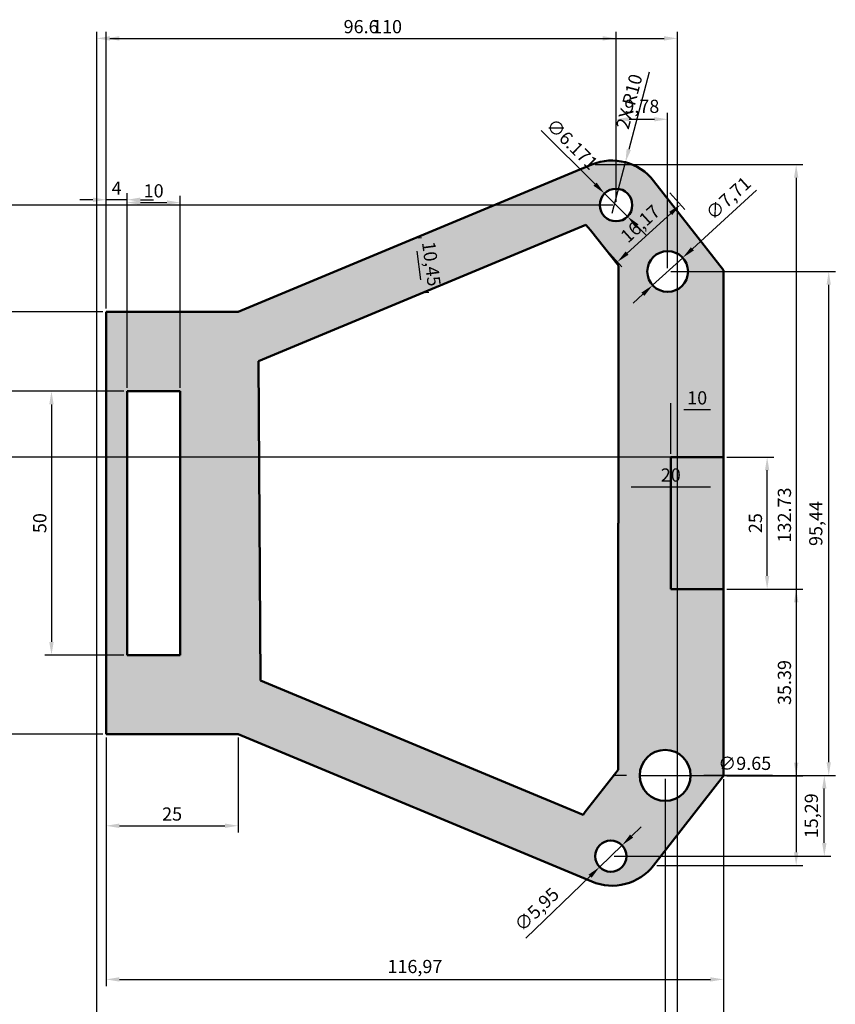
# Model space of a CAD drawing. Units: millimetres. Extents: x 2180 to 2428, y 1025 to 1371.
# Tile 3 of 3: x 2274 to 2428, y 1185 to 1371. Entities that reach past the tile are written whole.
import ezdxf

# ---------------------------------------------------------------- set-up
doc = ezdxf.new("R2010")
doc.units = ezdxf.units.MM
for name, color, linetype, lineweight in [('M-DIMS', 2, 'Continuous', 25), ('M-HATC', 252, 'Continuous', 18), ('M-OUTL', 7, 'Continuous', 50)]:
    doc.layers.add(name, color=color, linetype=linetype, lineweight=lineweight)
doc.styles.get("Standard").update_dxf_attribs({"font": 'arial.ttf'})
doc.dimstyles.new('ISO-25', dxfattribs={"dimtxt": 2.5, "dimasz": 2.5, "dimexe": 1.25, "dimexo": 0.625, "dimtad": 1, "dimtxsty": 'Standard', "dimcen": 2.5, "dimadec": 0, "dimazin": 0, "dimtfac": 1, "dimtmove": 0, "dimatfit": 3, "dimfxl": 1, "dimarcsym": 0})

# ---------------------------------------------------------------- blocks, each defined once
blk = doc.blocks.new('*D6')
at = {"layer": 'Defpoints', "color": 0, "transparency": 16777216}
for p in [(2290.36, 1316.12), (2266.28, 1236.12), (2290.36, 1236.12)]:
    blk.add_point(p, dxfattribs=at)
at = {"layer": 'M-DIMS', "color": 0, "lineweight": -2, "transparency": 16777216}
for p, q in [((2289.74, 1316.12), (2265.03, 1316.12)), ((2266.28, 1313.62), (2266.28, 1238.62)), ((2289.74, 1236.12), (2265.03, 1236.12))]:
    blk.add_line(p, q, dxfattribs=at)
at = {"layer": 'M-DIMS', "color": 0, "transparency": 16777216}
for points in [[(2265.87, 1313.62), (2266.7, 1313.62), (2266.28, 1316.12)], [(2265.87, 1238.62), (2266.7, 1238.62), (2266.28, 1236.12)]]:
    blk.add_solid(points, dxfattribs=at)
at = {"layer": 'M-DIMS', "color": 0, "transparency": 16777216, "insert": (2264.38, 1276.12), "char_height": 2.5, "attachment_point": 5, "rotation": 90}
blk.add_mtext('80', dxfattribs=at)
blk = doc.blocks.new('*D7')
at = {"layer": 'Defpoints', "color": 0, "transparency": 16777216}
for p in [(2294.36, 1301.12), (2280.01, 1251.12), (2294.36, 1251.12)]:
    blk.add_point(p, dxfattribs=at)
at = {"layer": 'M-DIMS', "color": 0, "lineweight": -2, "transparency": 16777216}
for p, q in [((2293.74, 1301.12), (2278.76, 1301.12)), ((2280.01, 1298.62), (2280.01, 1253.62)), ((2293.74, 1251.12), (2278.76, 1251.12))]:
    blk.add_line(p, q, dxfattribs=at)
at = {"layer": 'M-DIMS', "color": 0, "transparency": 16777216}
for points in [[(2279.59, 1298.62), (2280.42, 1298.62), (2280.01, 1301.12)], [(2279.59, 1253.62), (2280.42, 1253.62), (2280.01, 1251.12)]]:
    blk.add_solid(points, dxfattribs=at)
at = {"layer": 'M-DIMS', "color": 0, "transparency": 16777216, "insert": (2278.11, 1276.12), "char_height": 2.5, "attachment_point": 5, "rotation": 90}
blk.add_mtext('50', dxfattribs=at)
blk = doc.blocks.new('*D8')
at = {"layer": 'Defpoints', "color": 0, "transparency": 16777216}
for p in [(2290.36, 1337.37), (2290.36, 1316.12), (2294.36, 1301.12)]:
    blk.add_point(p, dxfattribs=at)
at = {"layer": 'M-DIMS', "color": 0, "lineweight": -2, "transparency": 16777216}
for p, q in [((2287.86, 1337.37), (2285.36, 1337.37)), ((2290.36, 1316.75), (2290.36, 1338.62)), ((2294.36, 1337.37), (2290.36, 1337.37)), ((2294.36, 1301.75), (2294.36, 1338.62)), ((2296.86, 1337.37), (2299.36, 1337.37))]:
    blk.add_line(p, q, dxfattribs=at)
at = {"layer": 'M-DIMS', "color": 0, "transparency": 16777216}
for points in [[(2287.86, 1337.79), (2287.86, 1336.95), (2290.36, 1337.37)], [(2296.86, 1337.79), (2296.86, 1336.95), (2294.36, 1337.37)]]:
    blk.add_solid(points, dxfattribs=at)
at = {"layer": 'M-DIMS', "color": 0, "transparency": 16777216, "insert": (2292.36, 1339.25), "char_height": 2.5, "attachment_point": 5}
blk.add_mtext('4', dxfattribs=at)
blk = doc.blocks.new('*D9')
at = {"layer": 'Defpoints', "color": 0, "transparency": 16777216}
for p in [(2304.36, 1336.83), (2294.36, 1301.12), (2304.36, 1301.12)]:
    blk.add_point(p, dxfattribs=at)
at = {"layer": 'M-DIMS', "color": 0, "lineweight": -2, "transparency": 16777216}
for p, q in [((2294.36, 1301.75), (2294.36, 1338.08)), ((2304.36, 1301.75), (2304.36, 1338.08)), ((2296.86, 1336.83), (2301.86, 1336.83))]:
    blk.add_line(p, q, dxfattribs=at)
at = {"layer": 'M-DIMS', "color": 0, "transparency": 16777216}
for points in [[(2296.86, 1337.25), (2296.86, 1336.42), (2294.36, 1336.83)], [(2301.86, 1337.25), (2301.86, 1336.42), (2304.36, 1336.83)]]:
    blk.add_solid(points, dxfattribs=at)
at = {"layer": 'M-DIMS', "color": 0, "transparency": 16777216, "insert": (2299.36, 1338.73), "char_height": 2.5, "attachment_point": 5}
blk.add_mtext('10', dxfattribs=at)
blk = doc.blocks.new('*D10')
at = {"layer": 'Defpoints', "color": 0, "transparency": 16777216}
for p in [(2348.86, 1330.08), (2350.25, 1319.72), (2350.25, 1319.72)]:
    blk.add_point(p, dxfattribs=at)
at = {"layer": 'M-DIMS', "color": 0, "lineweight": -2, "transparency": 16777216}
for p, q in [((2349.48, 1330.16), (2350.1, 1330.24)), ((2349.19, 1327.6), (2349.92, 1322.2)), ((2350.87, 1319.81), (2351.49, 1319.89))]:
    blk.add_line(p, q, dxfattribs=at)
at = {"layer": 'M-DIMS', "color": 0, "transparency": 16777216}
for points in [[(2349.61, 1327.65), (2348.78, 1327.54), (2348.86, 1330.08)], [(2350.33, 1322.26), (2349.5, 1322.14), (2350.25, 1319.72)]]:
    blk.add_solid(points, dxfattribs=at)
at = {"layer": 'M-DIMS', "color": 0, "transparency": 16777216, "insert": (2351.66, 1325.18), "char_height": 2.5, "attachment_point": 5, "rotation": 277.6268}
blk.add_mtext('10,45', dxfattribs=at)
blk = doc.blocks.new('*D11')
at = {"layer": 'Defpoints', "color": 0, "transparency": 16777216}
for p in [(2290.36, 1236.12), (2315.36, 1236.12), (2315.36, 1218.8)]:
    blk.add_point(p, dxfattribs=at)
at = {"layer": 'M-DIMS', "color": 0, "lineweight": -2, "transparency": 16777216}
for p, q in [((2290.36, 1235.5), (2290.36, 1217.55)), ((2315.36, 1235.5), (2315.36, 1217.55)), ((2292.86, 1218.8), (2312.86, 1218.8))]:
    blk.add_line(p, q, dxfattribs=at)
at = {"layer": 'M-DIMS', "color": 0, "transparency": 16777216}
for points in [[(2292.86, 1219.22), (2292.86, 1218.38), (2290.36, 1218.8)], [(2312.86, 1219.22), (2312.86, 1218.38), (2315.36, 1218.8)]]:
    blk.add_solid(points, dxfattribs=at)
at = {"layer": 'M-DIMS', "color": 0, "transparency": 16777216, "insert": (2302.86, 1220.7), "char_height": 2.5, "attachment_point": 5}
blk.add_mtext('25', dxfattribs=at)
blk = doc.blocks.new('*D12')
at = {"layer": 'Defpoints', "color": 0, "transparency": 16777216}
for p in [(2290.36, 1236.12), (2407.33, 1228.24), (2407.33, 1189.7)]:
    blk.add_point(p, dxfattribs=at)
at = {"layer": 'M-DIMS', "color": 0, "lineweight": -2, "transparency": 16777216}
for p, q in [((2290.36, 1235.5), (2290.36, 1188.45)), ((2407.33, 1227.61), (2407.33, 1188.45)), ((2292.86, 1189.7), (2404.83, 1189.7))]:
    blk.add_line(p, q, dxfattribs=at)
at = {"layer": 'M-DIMS', "color": 0, "transparency": 16777216}
for points in [[(2292.86, 1190.11), (2292.86, 1189.28), (2290.36, 1189.7)], [(2404.83, 1190.11), (2404.83, 1189.28), (2407.33, 1189.7)]]:
    blk.add_solid(points, dxfattribs=at)
at = {"layer": 'M-DIMS', "color": 0, "transparency": 16777216, "insert": (2348.85, 1191.82), "char_height": 2.5, "attachment_point": 5}
blk.add_mtext('116,97', dxfattribs=at)
blk = doc.blocks.new('*D13')
at = {"layer": 'Defpoints', "color": 0, "transparency": 16777216}
for p in [(2396.26, 1228.33), (2426.41, 1228.33), (2385.97, 1213.04)]:
    blk.add_point(p, dxfattribs=at)
at = {"layer": 'M-DIMS', "color": 0, "lineweight": -2, "transparency": 16777216}
for p, q in [((2396.89, 1228.33), (2427.66, 1228.33)), ((2426.41, 1215.54), (2426.41, 1225.83)), ((2386.59, 1213.04), (2427.66, 1213.04))]:
    blk.add_line(p, q, dxfattribs=at)
at = {"layer": 'M-DIMS', "color": 0, "transparency": 16777216}
for points in [[(2425.99, 1225.83), (2426.83, 1225.83), (2426.41, 1228.33)], [(2425.99, 1215.54), (2426.83, 1215.54), (2426.41, 1213.04)]]:
    blk.add_solid(points, dxfattribs=at)
at = {"layer": 'M-DIMS', "color": 0, "transparency": 16777216, "insert": (2424.28, 1220.69), "char_height": 2.5, "attachment_point": 5, "rotation": 90}
blk.add_mtext('15,29', dxfattribs=at)
blk = doc.blocks.new('*D14')
at = {"layer": 'Defpoints', "color": 0, "transparency": 16777216}
for p in [(2396.73, 1323.77), (2427.25, 1323.77), (2396.26, 1228.33)]:
    blk.add_point(p, dxfattribs=at)
at = {"layer": 'M-DIMS', "color": 0, "lineweight": -2, "transparency": 16777216}
for p, q in [((2397.36, 1323.77), (2428.5, 1323.77)), ((2427.25, 1230.83), (2427.25, 1321.27)), ((2396.89, 1228.33), (2428.5, 1228.33))]:
    blk.add_line(p, q, dxfattribs=at)
at = {"layer": 'M-DIMS', "color": 0, "transparency": 16777216}
for points in [[(2426.83, 1321.27), (2427.66, 1321.27), (2427.25, 1323.77)], [(2426.83, 1230.83), (2427.66, 1230.83), (2427.25, 1228.33)]]:
    blk.add_solid(points, dxfattribs=at)
at = {"layer": 'M-DIMS', "color": 0, "transparency": 16777216, "insert": (2425.12, 1276.05), "char_height": 2.5, "attachment_point": 5, "rotation": 90}
blk.add_mtext('95,44', dxfattribs=at)
blk = doc.blocks.new('*D15')
at = {"layer": 'Defpoints', "color": 0, "transparency": 16777216}
for p in [(2396.73, 1352.61), (2386.95, 1336.37), (2396.73, 1323.77)]:
    blk.add_point(p, dxfattribs=at)
at = {"layer": 'M-DIMS', "color": 0, "lineweight": -2, "transparency": 16777216}
for p, q in [((2386.95, 1337), (2386.95, 1353.86)), ((2389.45, 1352.61), (2394.23, 1352.61)), ((2396.73, 1324.4), (2396.73, 1353.86))]:
    blk.add_line(p, q, dxfattribs=at)
at = {"layer": 'M-DIMS', "color": 0, "transparency": 16777216}
for points in [[(2389.45, 1353.03), (2389.45, 1352.2), (2386.95, 1352.61)], [(2394.23, 1353.03), (2394.23, 1352.2), (2396.73, 1352.61)]]:
    blk.add_solid(points, dxfattribs=at)
at = {"layer": 'M-DIMS', "color": 0, "transparency": 16777216, "insert": (2391.84, 1354.74), "char_height": 2.5, "attachment_point": 5}
blk.add_mtext('9,78', dxfattribs=at)
blk = doc.blocks.new('*D16')
at = {"layer": 'Defpoints', "color": 0, "transparency": 16777216}
for p in [(2399.58, 1326.38), (2393.89, 1321.17)]:
    blk.add_point(p, dxfattribs=at)
at = {"layer": 'M-DIMS', "color": 0, "lineweight": -2, "transparency": 16777216}
for p, q in [((2413.59, 1339.2), (2401.42, 1328.06)), ((2393.89, 1321.17), (2399.58, 1326.38)), ((2392.04, 1319.48), (2390.2, 1317.79))]:
    blk.add_line(p, q, dxfattribs=at)
at = {"layer": 'M-DIMS', "color": 0, "transparency": 16777216}
for points in [[(2401.14, 1328.37), (2401.7, 1327.76), (2399.58, 1326.38)], [(2391.76, 1319.79), (2392.33, 1319.17), (2393.89, 1321.17)]]:
    blk.add_solid(points, dxfattribs=at)
at = {"layer": 'M-DIMS', "color": 0, "transparency": 16777216, "insert": (2408.44, 1337.43), "char_height": 2.5, "attachment_point": 5, "rotation": 42.4638}
blk.add_mtext('∅7,71', dxfattribs=at)
blk = doc.blocks.new('*D17')
at = {"layer": 'Defpoints', "color": 0, "transparency": 16777216}
for p in [(2388.11, 1215.11), (2383.83, 1210.98)]:
    blk.add_point(p, dxfattribs=at)
at = {"layer": 'M-DIMS', "color": 0, "lineweight": -2, "transparency": 16777216}
for p, q in [((2389.9, 1216.84), (2391.7, 1218.58)), ((2388.11, 1215.11), (2383.83, 1210.98)), ((2369.88, 1197.52), (2382.03, 1209.24))]:
    blk.add_line(p, q, dxfattribs=at)
at = {"layer": 'M-DIMS', "color": 0, "transparency": 16777216}
for points in [[(2389.61, 1217.14), (2390.19, 1216.54), (2388.11, 1215.11)], [(2381.74, 1209.54), (2382.32, 1208.94), (2383.83, 1210.98)]]:
    blk.add_solid(points, dxfattribs=at)
at = {"layer": 'M-DIMS', "color": 0, "transparency": 16777216, "insert": (2372.15, 1202.72), "char_height": 2.5, "attachment_point": 5, "rotation": 43.9913}
blk.add_mtext('∅5,95', dxfattribs=at)
blk = doc.blocks.new('*D18')
at = {"layer": 'Defpoints', "color": 0, "transparency": 16777216}
for p in [(2407.33, 1283.01), (2387.33, 1276.12), (2407.33, 1276.12)]:
    blk.add_point(p, dxfattribs=at)
at = {"layer": 'M-DIMS', "color": 0, "lineweight": -2, "transparency": 16777216}
for p, q in [((2387.33, 1276.75), (2387.33, 1284.26)), ((2407.33, 1276.75), (2407.33, 1284.26)), ((2389.83, 1283.01), (2404.83, 1283.01))]:
    blk.add_line(p, q, dxfattribs=at)
at = {"layer": 'M-DIMS', "color": 0, "transparency": 16777216}
for points in [[(2389.83, 1283.42), (2389.83, 1282.59), (2387.33, 1283.01)], [(2404.83, 1283.42), (2404.83, 1282.59), (2407.33, 1283.01)]]:
    blk.add_solid(points, dxfattribs=at)
at = {"layer": 'M-DIMS', "color": 0, "transparency": 16777216, "insert": (2397.33, 1284.91), "char_height": 2.5, "attachment_point": 5}
blk.add_mtext('20', dxfattribs=at)
blk = doc.blocks.new('*D19')
at = {"layer": 'Defpoints', "color": 0, "transparency": 16777216}
for p in [(2396.73, 1339.13), (2399.16, 1336.46), (2384.77, 1328.26)]:
    blk.add_point(p, dxfattribs=at)
at = {"layer": 'M-DIMS', "color": 0, "lineweight": -2, "transparency": 16777216}
for p, q in [((2397.15, 1338.67), (2400, 1335.53)), ((2389.05, 1327.27), (2397.31, 1334.78)), ((2385.19, 1327.79), (2388.04, 1324.66))]:
    blk.add_line(p, q, dxfattribs=at)
at = {"layer": 'M-DIMS', "color": 0, "transparency": 16777216}
for points in [[(2397.03, 1335.08), (2397.59, 1334.47), (2399.16, 1336.46)], [(2388.77, 1327.57), (2389.33, 1326.96), (2387.2, 1325.58)]]:
    blk.add_solid(points, dxfattribs=at)
at = {"layer": 'M-DIMS', "color": 0, "transparency": 16777216, "insert": (2391.75, 1332.59), "char_height": 2.5, "attachment_point": 5, "rotation": 42.2758}
blk.add_mtext('16,17', dxfattribs=at)
blk = doc.blocks.new('*D20')
at = {"layer": 'Defpoints', "color": 0, "transparency": 16777216}
for p in [(2407.33, 1288.62), (2415.58, 1288.62), (2407.33, 1263.62)]:
    blk.add_point(p, dxfattribs=at)
at = {"layer": 'M-DIMS', "color": 0, "lineweight": -2, "transparency": 16777216}
for p, q in [((2407.96, 1288.62), (2416.83, 1288.62)), ((2415.58, 1266.12), (2415.58, 1286.12)), ((2407.96, 1263.62), (2416.83, 1263.62))]:
    blk.add_line(p, q, dxfattribs=at)
at = {"layer": 'M-DIMS', "color": 0, "transparency": 16777216}
for points in [[(2415.16, 1286.12), (2415.99, 1286.12), (2415.58, 1288.62)], [(2415.16, 1266.12), (2415.99, 1266.12), (2415.58, 1263.62)]]:
    blk.add_solid(points, dxfattribs=at)
at = {"layer": 'M-DIMS', "color": 0, "transparency": 16777216, "insert": (2413.68, 1276.12), "char_height": 2.5, "attachment_point": 5, "rotation": 90}
blk.add_mtext('25', dxfattribs=at)
blk = doc.blocks.new('*D21')
at = {"layer": 'Defpoints', "color": 0, "transparency": 16777216}
for p in [(2407.33, 1297.62), (2397.33, 1288.62), (2407.33, 1288.62)]:
    blk.add_point(p, dxfattribs=at)
at = {"layer": 'M-DIMS', "color": 0, "lineweight": -2, "transparency": 16777216}
for p, q in [((2397.33, 1289.25), (2397.33, 1298.87)), ((2407.33, 1289.25), (2407.33, 1298.87)), ((2399.83, 1297.62), (2404.83, 1297.62))]:
    blk.add_line(p, q, dxfattribs=at)
at = {"layer": 'M-DIMS', "color": 0, "transparency": 16777216}
for points in [[(2399.83, 1298.04), (2399.83, 1297.2), (2397.33, 1297.62)], [(2404.83, 1298.04), (2404.83, 1297.2), (2407.33, 1297.62)]]:
    blk.add_solid(points, dxfattribs=at)
at = {"layer": 'M-DIMS', "color": 0, "transparency": 16777216, "insert": (2402.33, 1299.52), "char_height": 2.5, "attachment_point": 5}
blk.add_mtext('10', dxfattribs=at)
blk = doc.blocks.new('*D35')
at = {"layer": 'Defpoints', "color": 0, "transparency": 16777216}
for p in [(2386.95, 1367.93), (2386.95, 1336.37), (2290.36, 1316.12)]:
    blk.add_point(p, dxfattribs=at)
at = {"layer": 'M-DIMS', "color": 0, "lineweight": -2, "transparency": 16777216}
for p, q in [((2290.36, 1316.75), (2290.36, 1369.18)), ((2386.95, 1337), (2386.95, 1369.18)), ((2292.86, 1367.93), (2384.45, 1367.93))]:
    blk.add_line(p, q, dxfattribs=at)
at = {"layer": 'M-DIMS', "color": 0, "transparency": 16777216}
for points in [[(2292.86, 1368.35), (2292.86, 1367.51), (2290.36, 1367.93)], [(2384.45, 1368.35), (2384.45, 1367.51), (2386.95, 1367.93)]]:
    blk.add_solid(points, dxfattribs=at)
at = {"layer": 'M-DIMS', "color": 0, "transparency": 16777216, "insert": (2338.66, 1369.83), "char_height": 2.5, "attachment_point": 5}
blk.add_mtext('96.6', dxfattribs=at)
blk = doc.blocks.new('*D36')
at = {"layer": 'Defpoints', "color": 0, "transparency": 16777216}
for p in [(2386.95, 1336.37), (2187.07, 1288.62), (2407.33, 1288.62)]:
    blk.add_point(p, dxfattribs=at)
at = {"layer": 'M-DIMS', "color": 0, "lineweight": -2, "transparency": 16777216}
for p, q in [((2386.33, 1336.37), (2185.82, 1336.37)), ((2187.07, 1333.87), (2187.07, 1291.12)), ((2406.71, 1288.62), (2185.82, 1288.62))]:
    blk.add_line(p, q, dxfattribs=at)
at = {"layer": 'M-DIMS', "color": 0, "transparency": 16777216}
for points in [[(2186.65, 1333.87), (2187.49, 1333.87), (2187.07, 1336.37)], [(2186.65, 1291.12), (2187.49, 1291.12), (2187.07, 1288.62)]]:
    blk.add_solid(points, dxfattribs=at)
at = {"layer": 'M-DIMS', "color": 0, "transparency": 16777216, "insert": (2185.17, 1312.5), "char_height": 2.5, "attachment_point": 5, "rotation": 90}
blk.add_mtext('47.75', dxfattribs=at)
blk = doc.blocks.new('*D37')
at = {"layer": 'Defpoints', "color": 0, "transparency": 16777216}
for p in [(2396.26, 1228.33), (2407.33, 1228.24), (2407.33, 1089.54)]:
    blk.add_point(p, dxfattribs=at)
at = {"layer": 'M-DIMS', "color": 0, "lineweight": -2, "transparency": 16777216}
for p, q in [((2396.26, 1227.71), (2396.26, 1088.29)), ((2407.33, 1227.61), (2407.33, 1088.29)), ((2398.76, 1089.54), (2404.83, 1089.54))]:
    blk.add_line(p, q, dxfattribs=at)
at = {"layer": 'M-DIMS', "color": 0, "transparency": 16777216}
for points in [[(2398.76, 1089.96), (2398.76, 1089.12), (2396.26, 1089.54)], [(2404.83, 1089.96), (2404.83, 1089.12), (2407.33, 1089.54)]]:
    blk.add_solid(points, dxfattribs=at)
at = {"layer": 'M-DIMS', "color": 0, "transparency": 16777216, "insert": (2401.8, 1091.44), "char_height": 2.5, "attachment_point": 5}
blk.add_mtext('11.07', dxfattribs=at)
blk = doc.blocks.new('*D38')
at = {"layer": 'Defpoints', "color": 0, "transparency": 16777216}
for p in [(2407.33, 1263.62), (2407.33, 1228.24), (2421.08, 1228.24)]:
    blk.add_point(p, dxfattribs=at)
at = {"layer": 'M-DIMS', "color": 0, "lineweight": -2, "transparency": 16777216}
for p, q in [((2407.96, 1263.62), (2422.33, 1263.62)), ((2421.08, 1261.12), (2421.08, 1230.74)), ((2407.96, 1228.24), (2422.33, 1228.24))]:
    blk.add_line(p, q, dxfattribs=at)
at = {"layer": 'M-DIMS', "color": 0, "transparency": 16777216}
for points in [[(2420.67, 1261.12), (2421.5, 1261.12), (2421.08, 1263.62)], [(2420.67, 1230.74), (2421.5, 1230.74), (2421.08, 1228.24)]]:
    blk.add_solid(points, dxfattribs=at)
at = {"layer": 'M-DIMS', "color": 0, "transparency": 16777216, "insert": (2419.18, 1245.93), "char_height": 2.5, "attachment_point": 5, "rotation": 90}
blk.add_mtext('35.39', dxfattribs=at)
blk = doc.blocks.new('*D39')
at = {"layer": 'Defpoints', "color": 0, "transparency": 16777216}
for p in [(2382.36, 1344.03), (2394.08, 1211.29), (2421.08, 1211.29)]:
    blk.add_point(p, dxfattribs=at)
at = {"layer": 'M-DIMS', "color": 0, "lineweight": -2, "transparency": 16777216}
for p, q in [((2382.99, 1344.03), (2422.33, 1344.03)), ((2421.08, 1341.53), (2421.08, 1213.79)), ((2394.71, 1211.29), (2422.33, 1211.29))]:
    blk.add_line(p, q, dxfattribs=at)
at = {"layer": 'M-DIMS', "color": 0, "transparency": 16777216}
for points in [[(2420.67, 1341.53), (2421.5, 1341.53), (2421.08, 1344.03)], [(2420.67, 1213.79), (2421.5, 1213.79), (2421.08, 1211.29)]]:
    blk.add_solid(points, dxfattribs=at)
at = {"layer": 'M-DIMS', "color": 0, "transparency": 16777216, "insert": (2419.18, 1277.66), "char_height": 2.5, "attachment_point": 5, "rotation": 90}
blk.add_mtext('132.73', dxfattribs=at)
blk = doc.blocks.new('*D40')
at = {"layer": 'Defpoints', "color": 0, "transparency": 16777216}
for p in [(2290.36, 1316.12), (2187.07, 1301.12), (2294.36, 1301.12)]:
    blk.add_point(p, dxfattribs=at)
at = {"layer": 'M-DIMS', "color": 0, "lineweight": -2, "transparency": 16777216}
for p, q in [((2289.74, 1316.12), (2185.82, 1316.12)), ((2187.07, 1313.62), (2187.07, 1303.62)), ((2293.74, 1301.12), (2185.82, 1301.12))]:
    blk.add_line(p, q, dxfattribs=at)
at = {"layer": 'M-DIMS', "color": 0, "transparency": 16777216}
for points in [[(2186.65, 1313.62), (2187.49, 1313.62), (2187.07, 1316.12)], [(2186.65, 1303.62), (2187.49, 1303.62), (2187.07, 1301.12)]]:
    blk.add_solid(points, dxfattribs=at)
at = {"layer": 'M-DIMS', "color": 0, "transparency": 16777216, "insert": (2185.17, 1308.62), "char_height": 2.5, "attachment_point": 5, "rotation": 90}
blk.add_mtext('15', dxfattribs=at)
blk = doc.blocks.new('*D41')
at = {"layer": 'Defpoints', "color": 0, "transparency": 16777216}
for p in [(2398.57, 1367.93), (2288.57, 1149.5), (2398.57, 1149.5)]:
    blk.add_point(p, dxfattribs=at)
at = {"layer": 'M-DIMS', "color": 0, "lineweight": -2, "transparency": 16777216}
for p, q in [((2288.57, 1150.12), (2288.57, 1369.18)), ((2398.57, 1150.12), (2398.57, 1369.18)), ((2291.07, 1367.93), (2396.07, 1367.93))]:
    blk.add_line(p, q, dxfattribs=at)
at = {"layer": 'M-DIMS', "color": 0, "transparency": 16777216}
for points in [[(2291.07, 1368.35), (2291.07, 1367.51), (2288.57, 1367.93)], [(2396.07, 1368.35), (2396.07, 1367.51), (2398.57, 1367.93)]]:
    blk.add_solid(points, dxfattribs=at)
at = {"layer": 'M-DIMS', "color": 0, "transparency": 16777216, "insert": (2343.57, 1369.83), "char_height": 2.5, "attachment_point": 5}
blk.add_mtext('110', dxfattribs=at)
blk = doc.blocks.new('*D48')
at = {"layer": 'Defpoints', "color": 0, "transparency": 16777216}
for p in [(2388.74, 1344.47), (2386.21, 1334.8)]:
    blk.add_point(p, dxfattribs=at)
at = {"layer": 'M-DIMS', "color": 0, "lineweight": -2, "transparency": 16777216}
for p, q in [((2393.21, 1361.52), (2389.37, 1346.89)), ((2386.21, 1334.8), (2388.74, 1344.47))]:
    blk.add_line(p, q, dxfattribs=at)
at = {"layer": 'M-DIMS', "color": 0, "transparency": 16777216}
blk.add_solid([(2388.97, 1346.99), (2389.78, 1346.78), (2388.74, 1344.47)], dxfattribs=at)
at = {"layer": 'M-DIMS', "color": 0, "transparency": 16777216, "insert": (2389.77, 1355.9), "char_height": 2.5, "attachment_point": 5, "rotation": 75.3136}
blk.add_mtext('2X R10', dxfattribs=at)
blk = doc.blocks.new('*D49')
at = {"layer": 'Defpoints', "color": 0, "transparency": 16777216}
for p in [(2391.44, 1228.33), (2401.09, 1228.33)]:
    blk.add_point(p, dxfattribs=at)
at = {"layer": 'M-DIMS', "color": 0, "lineweight": -2, "transparency": 16777216}
for p, q in [((2388.94, 1228.33), (2386.44, 1228.33)), ((2391.44, 1228.33), (2401.09, 1228.33)), ((2416.57, 1228.33), (2403.59, 1228.33))]:
    blk.add_line(p, q, dxfattribs=at)
at = {"layer": 'M-DIMS', "color": 0, "transparency": 16777216}
for points in [[(2388.94, 1228.75), (2388.94, 1227.91), (2391.44, 1228.33)], [(2403.59, 1228.75), (2403.59, 1227.91), (2401.09, 1228.33)]]:
    blk.add_solid(points, dxfattribs=at)
at = {"layer": 'M-DIMS', "color": 0, "transparency": 16777216, "insert": (2411.33, 1230.3), "char_height": 2.5, "attachment_point": 5, "rotation": 359.9984}
blk.add_mtext('∅9.65', dxfattribs=at)
blk = doc.blocks.new('*D50')
at = {"layer": 'Defpoints', "color": 0, "transparency": 16777216}
for p in [(2384.77, 1338.55), (2389.14, 1334.19)]:
    blk.add_point(p, dxfattribs=at)
at = {"layer": 'M-DIMS', "color": 0, "lineweight": -2, "transparency": 16777216}
for p, q in [((2372.79, 1350.5), (2383, 1340.32)), ((2389.14, 1334.19), (2384.77, 1338.55)), ((2390.91, 1332.43), (2392.68, 1330.66))]:
    blk.add_line(p, q, dxfattribs=at)
at = {"layer": 'M-DIMS', "color": 0, "transparency": 16777216}
for points in [[(2383.29, 1340.61), (2382.7, 1340.02), (2384.77, 1338.55)], [(2391.2, 1332.72), (2390.61, 1332.13), (2389.14, 1334.19)]]:
    blk.add_solid(points, dxfattribs=at)
at = {"layer": 'M-DIMS', "color": 0, "transparency": 16777216, "insert": (2378.4, 1347.69), "char_height": 2.5, "attachment_point": 5, "rotation": 315.0756}
blk.add_mtext('∅6.171', dxfattribs=at)

msp = doc.modelspace()

# ---------------------------------------------------------------- hatches: boundary and pattern name
at = {"layer": 'M-HATC'}
h = msp.add_hatch(color=256, dxfattribs=at)
h.set_gradient(color1=(100, 33, 101), color2=(100, 33, 101), tint=1)
h.paths.add_polyline_path([(2290.3614, 1316.125), (2290.3614, 1236.125), (2315.3614, 1236.125), (2382.3613, 1208.2225, 0.33744335), (2394.0834, 1211.2942), (2407.3324, 1228.2381), (2407.3324, 1276.125), (2407.3324, 1324.0118), (2394.0834, 1340.9557, 0.33744335), (2382.3613, 1344.0274), (2315.3614, 1316.125)])
h.paths.add_polyline_path([(2304.3614, 1301.125), (2304.3614, 1251.125), (2294.3614, 1251.125), (2294.3614, 1301.125)], flags=16)
h.paths.add_polyline_path([(2319.2409, 1306.8094), (2381.2546, 1332.6353), (2382.1426, 1331.6188), (2387.4019, 1324.8927), (2387.4019, 1324.0118), (2387.4019, 1276.125), (2387.3338, 1229.3759), (2381.1207, 1221.4302), (2380.7182, 1220.8933), (2319.6154, 1246.3398)], flags=16)
h.paths.add_polyline_path([(2383.8679, 1336.3721, -1), (2390.0393, 1336.3721, -1)], flags=16)
h.paths.add_polyline_path([(2392.8764, 1323.7723, -1), (2400.5906, 1323.7723, -1)], flags=16)
h.paths.add_polyline_path([(2401.0881, 1228.3311, -1), (2391.4386, 1228.3311, -1)], flags=16)
h.paths.add_polyline_path([(2388.94, 1213.0425, -1), (2382.9912, 1213.0425, -1)], flags=16)

# ---------------------------------------------------------------- linework, layer by layer
at = {"layer": 'M-OUTL'}
for p, q in [((2315.3614, 1316.125), (2382.3613, 1344.0274)), ((2394.0834, 1340.9557), (2407.3324, 1324.0118)), ((2319.2409, 1306.8094), (2381.2546, 1332.6353)), ((2382.1426, 1331.6188), (2381.2546, 1332.6353)), ((2382.1426, 1331.6188), (2387.4019, 1324.8927)), ((2387.4019, 1324.0118), (2387.4019, 1324.8927)), ((2387.4019, 1324.0118), (2387.4019, 1276.125)), ((2407.3324, 1324.0118), (2407.3324, 1276.125)), ((2290.3614, 1316.125), (2290.3614, 1236.125)), ((2290.3614, 1316.125), (2315.3614, 1316.125)), ((2319.2409, 1306.8094), (2319.6154, 1246.3398)), ((2294.3614, 1301.125), (2294.3614, 1251.125)), ((2304.3614, 1301.125), (2294.3614, 1301.125)), ((2304.3614, 1251.125), (2304.3614, 1301.125)), ((2407.3324, 1288.625), (2397.3324, 1288.625)), ((2397.3324, 1288.625), (2397.3324, 1263.625)), ((2407.3324, 1276.125), (2407.3324, 1288.625)), ((2387.3338, 1229.3759), (2387.3338, 1276.125)), ((2407.3324, 1228.2381), (2407.3324, 1276.125)), ((2397.3324, 1263.625), (2407.3324, 1263.625)), ((2294.3614, 1251.125), (2304.3614, 1251.125)), ((2319.6154, 1246.3398), (2380.7182, 1220.8933)), ((2290.3614, 1236.125), (2315.3614, 1236.125)), ((2315.3614, 1236.125), (2382.3613, 1208.2225)), ((2381.1207, 1221.4302), (2387.3338, 1229.3759)), ((2394.0834, 1211.2942), (2407.3324, 1228.2381)), ((2381.1207, 1221.4302), (2380.7182, 1220.8933))]:
    msp.add_line(p, q, dxfattribs=at)
for centre, radius in [((2386.9536, 1336.3721), 3.0857), ((2396.7335, 1323.7723), 3.8571), ((2396.2634, 1228.3311), 4.8247), ((2385.9656, 1213.0425), 2.9744)]:
    msp.add_circle(centre, radius, dxfattribs=at)
for centre, start, end in [((2386.2058, 1334.7959), 38.023033, 112.609533), ((2386.2058, 1217.454), 247.390467, 321.976967)]:
    msp.add_arc(centre, 10, start, end, dxfattribs=at)

# ---------------------------------------------------------------- dimensions: what is measured, and where the dimension line sits
at = {"layer": 'M-DIMS'}
for base, p1, p2, override, picture, middle in [((2398.5713, 1367.9295), (2288.5713, 1149.4968), (2398.5713, 1149.4968), {"dimdec": 0, "dimlfac": 1, "dimrnd": 0, "dimzin": 0, "dimdsep": 46, "dimlunit": 2}, '*D41', (2343.5713, 1369.831)), ((2386.9536, 1367.9295), (2290.3614, 1316.125), (2386.9536, 1336.3721), {"dimdec": 1, "dimlfac": 1, "dimrnd": 0, "dimzin": 0, "dimdsep": 46, "dimlunit": 2}, '*D35', (2338.6575, 1369.831)), ((2396.7335, 1352.6134), (2386.9536, 1336.3721), (2396.7335, 1323.7723), {"dimclrd": 0, "dimclre": 0, "dimclrt": 0}, '*D15', (2391.8435, 1354.7408)), ((2290.3614, 1337.3704), (2294.3614, 1301.125), (2290.3614, 1316.125), {"dimclrd": 0, "dimclre": 0, "dimclrt": 0}, '*D8', (2292.3614, 1339.2454)), ((2304.3614, 1336.8327), (2294.3614, 1301.125), (2304.3614, 1301.125), {"dimclrd": 0, "dimclre": 0, "dimclrt": 0}, '*D9', (2299.3614, 1338.7341)), ((2407.3324, 1297.6208), (2397.3324, 1288.625), (2407.3324, 1288.625), {"dimclrd": 0, "dimclre": 0, "dimclrt": 0}, '*D21', (2402.3324, 1299.5222)), ((2407.3324, 1283.0054), (2387.3338, 1276.125), (2407.3324, 1276.125), {"dimclrd": 0, "dimclre": 0, "dimclrt": 0}, '*D18', (2397.3331, 1284.9068)), ((2315.3614, 1218.7999), (2290.3614, 1236.125), (2315.3614, 1236.125), {"dimclrd": 0, "dimclre": 0, "dimclrt": 0}, '*D11', (2302.8614, 1220.7014)), ((2407.3324, 1189.6956), (2290.3614, 1236.125), (2407.3324, 1228.2381), {"dimclrd": 0, "dimclre": 0, "dimclrt": 0}, '*D12', (2348.8469, 1191.823)), ((2407.3324, 1089.5404), (2396.2634, 1228.3311), (2407.3324, 1228.2381), {"dimdec": 2, "dimlfac": 1, "dimrnd": 0, "dimzin": 0, "dimdsep": 46, "dimlunit": 2}, '*D37', (2401.7979, 1091.4418))]:
    dim = msp.add_linear_dim(base=base, p1=p1, p2=p2, dimstyle='ISO-25', override=override, dxfattribs=at)
    dim.commit()
    dim.dimension.update_dxf_attribs({"geometry": picture, "text_midpoint": middle})
dim = msp.add_radius_dim(center=(2386.2058, 1334.7959), mpoint=(2388.7411, 1344.4692), text='2X <>', dimstyle='ISO-25', override={"dimdec": 0, "dimlfac": 1, "dimrnd": 0, "dimzin": 0, "dimdsep": 46, "dimlunit": 2}, dxfattribs=at)
dim.commit()
dim.dimension.update_dxf_attribs({"geometry": '*D48', "text_midpoint": (2389.7704, 1355.8964)})
for p1, p2, override, picture, middle in [((2389.1384, 1334.1931), (2384.7688, 1338.5512), {"dimdec": 3, "dimlfac": 1, "dimrnd": 0, "dimzin": 0, "dimdsep": 46, "dimlunit": 2}, '*D50', (2377.0074, 1346.2921)), ((2393.8881, 1321.1683), (2399.5789, 1326.3763), {"dimclrd": 0, "dimclre": 0, "dimclrt": 0}, '*D16', (2409.907, 1335.8283)), ((2388.1055, 1215.1084), (2383.8257, 1210.9766), {"dimclrd": 0, "dimclre": 0, "dimclrt": 0}, '*D17', (2373.6524, 1201.1555))]:
    dim = msp.add_diameter_dim_2p(p1=p1, p2=p2, dimstyle='ISO-25', override=override, dxfattribs=at)
    dim.commit()
    dim.dimension.update_dxf_attribs({"geometry": picture, "text_midpoint": middle, "dimtype": 163})
for base, p1, p2, override, picture, middle in [((2421.0824, 1211.2942), (2382.3613, 1344.0274), (2394.0834, 1211.2942), {"dimdec": 2, "dimlfac": 1, "dimrnd": 0, "dimzin": 0, "dimdsep": 46, "dimlunit": 2}, '*D39', (2419.1801, 1277.6608)), ((2187.0692, 1288.625), (2386.9536, 1336.3721), (2407.3324, 1288.625), {"dimdec": 2, "dimlfac": 1, "dimrnd": 0, "dimzin": 0, "dimdsep": 46, "dimlunit": 2}, '*D36', (2185.1728, 1312.4986)), ((2427.2451, 1323.7723), (2396.2634, 1228.3311), (2396.7335, 1323.7723), {"dimclrd": 0, "dimclre": 0, "dimclrt": 0}, '*D14', (2425.1177, 1276.0517)), ((2187.0692, 1301.125), (2290.3614, 1316.125), (2294.3614, 1301.125), {"dimdec": 0, "dimlfac": 1, "dimrnd": 0, "dimzin": 0, "dimdsep": 46, "dimlunit": 2}, '*D40', (2185.1677, 1308.625)), ((2266.283, 1236.125), (2290.3614, 1316.125), (2290.3614, 1236.125), {"dimclrd": 0, "dimclre": 0, "dimclrt": 0}, '*D6', (2264.3816, 1276.125)), ((2280.0073, 1251.125), (2294.3614, 1301.125), (2294.3614, 1251.125), {"dimclrd": 0, "dimclre": 0, "dimclrt": 0}, '*D7', (2278.1058, 1276.125)), ((2415.5769, 1288.625), (2407.3324, 1263.625), (2407.3324, 1288.625), {"dimclrd": 0, "dimclre": 0, "dimclrt": 0}, '*D20', (2413.6754, 1276.125)), ((2421.0824, 1228.2381), (2407.3324, 1263.625), (2407.3324, 1228.2381), {"dimdec": 2, "dimlfac": 1, "dimrnd": 0, "dimzin": 0, "dimdsep": 46, "dimlunit": 2}, '*D38', (2419.1801, 1245.9316)), ((2426.4097, 1228.3311), (2385.9656, 1213.0425), (2396.2634, 1228.3311), {"dimclrd": 0, "dimclre": 0, "dimclrt": 0}, '*D13', (2424.2823, 1220.6868))]:
    dim = msp.add_linear_dim(base=base, p1=p1, p2=p2, angle=90, dimstyle='ISO-25', override=override, dxfattribs=at)
    dim.commit()
    dim.dimension.update_dxf_attribs({"geometry": picture, "text_midpoint": middle})
for p1, p2, distance, picture, middle in [((2384.7722, 1328.2557), (2396.7335, 1339.1304), -3.6116, '*D19', (2391.7513, 1332.5948)), ((2348.8613, 1330.0762), (2350.2478, 1319.7223), 0, '*D10', (2351.6631, 1325.1816))]:
    dim = msp.add_aligned_dim(p1=p1, p2=p2, distance=distance, dimstyle='ISO-25', override={"dimclrd": 0, "dimclre": 0, "dimclrt": 0}, dxfattribs=at)
    dim.commit()
    dim.dimension.update_dxf_attribs({"geometry": picture, "text_midpoint": middle})
dim = msp.add_diameter_dim_2p(p1=(2391.4386, 1228.3313), p2=(2401.0881, 1228.331), dimstyle='ISO-25', override={"dimdec": 2, "dimlfac": 1, "dimrnd": 0, "dimzin": 0, "dimdsep": 46, "dimlunit": 2}, dxfattribs=at)
dim.commit()
dim.dimension.update_dxf_attribs({"geometry": '*D49', "text_midpoint": (2411.3294, 1228.3307)})

doc.saveas('drawing.dxf')
